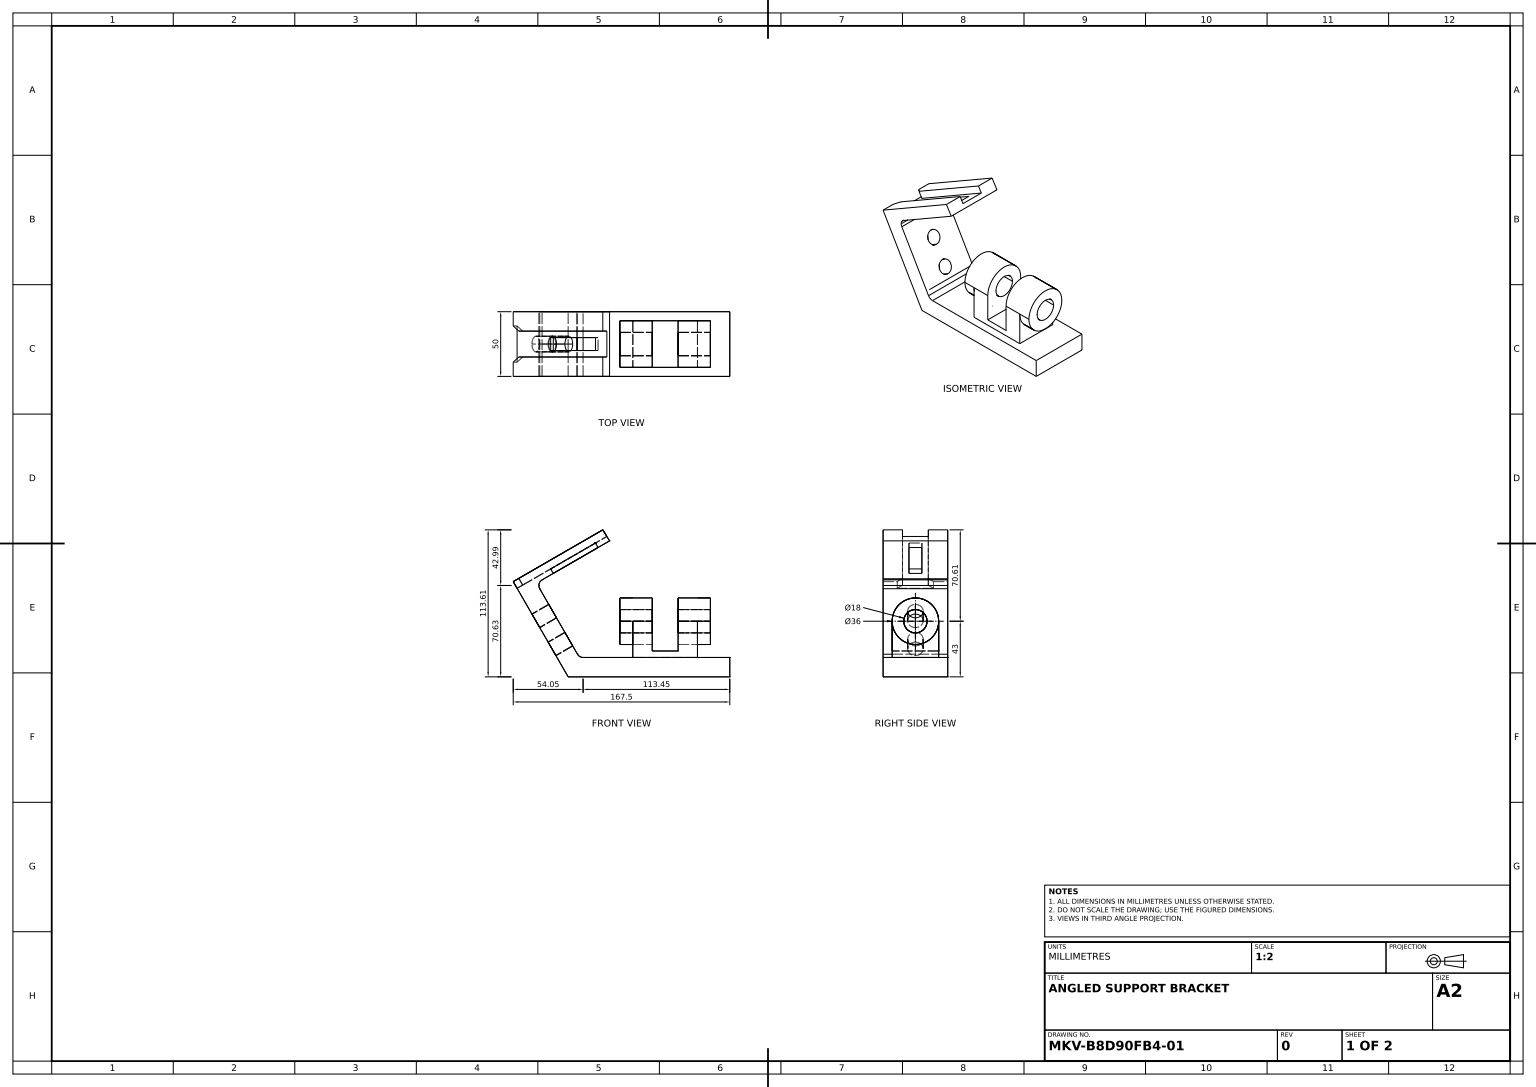
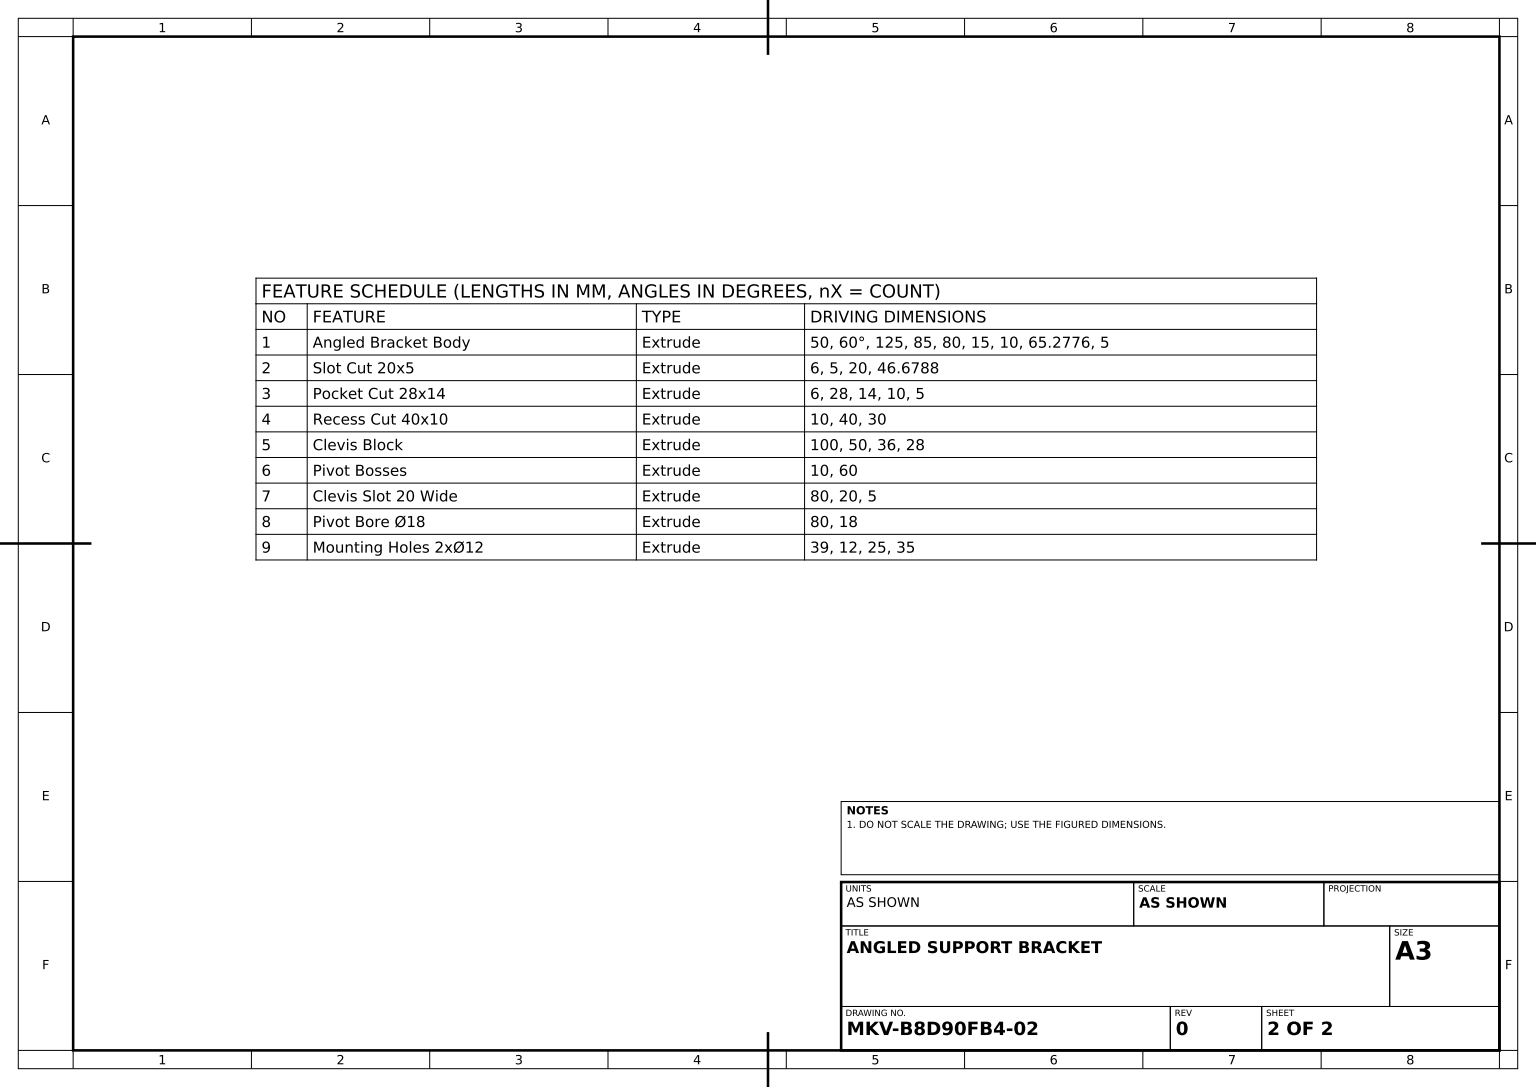
from build123d import *

# Parameters (mm, degrees)
ANGLED_BRACKET_BODY_DEPTH  = 25
SLOT_20X5_SKETCH_W         = 83.357534166
SLOT_20X5_SKETCH_H         = 20
SLOT_CUT_20X5_DEPTH        = 6
POCKET_CUT_28X14_DEPTH     = 6
RECESS_40X10_SKETCH_W      = 40
RECESS_40X10_SKETCH_H      = 10
RECESS_CUT_40X10_DEPTH     = 10
CLEVIS_BLOCK_SKETCH_W      = 36
CLEVIS_BLOCK_SKETCH_H      = 28
CLEVIS_BLOCK_DEPTH         = 50
PIVOT_BOSSES_DEPTH         = 10
PIVOT_BOSSES_DEPTH_BACK    = 60
PIVOT_BOSS_SKETCH_R        = 18
CLEVIS_SLOT_SKETCH_W       = 20
CLEVIS_SLOT_SKETCH_H       = 46
CLEVIS_SLOT_20_WIDE_DEPTH  = 80
PIVOT_BORE_SKETCH_R        = 9
PIVOT_BORE_18_DEPTH        = 80
MOUNTING_HOLES_SKETCH_R    = 6
MOUNTING_HOLES_2X_12_DEPTH = 39


with BuildPart() as part:
    # Bracket Profile Sketch → Angled Bracket Body (new, symmetric)
    with BuildSketch(Plane.XY):
        with BuildLine():
            Line((125, 0), (0, 0))
            Line((0, 0), (-42.5, 73.612159322))
            Line((-42.5, 73.612159322), (26.782032303, 113.612159322))
            Line((26.782032303, 113.612159322), (32.020529704, 105.094052432))
            Line((32.020529704, 105.094052432), (-20.181419095, 74.955243241))
            ThreePointArc((-20.181419095, 74.955243241), (-22.511048226, 71.919211448), (-22.011546114, 68.125116222))
            Line((-22.011546114, 68.125116222), (7.216878365, 17.5))
            ThreePointArc((7.216878365, 17.5), (9.047005384, 15.669872981), (11.547005384, 15))
            Line((11.547005384, 15), (125, 15))
            Line((125, 15), (125, 0))
        make_face()
    extrude(amount=ANGLED_BRACKET_BODY_DEPTH, both=True)

    # Slot 20x5 Sketch → Slot Cut 20x5 (cut)
    with BuildSketch(Plane(origin=(-42.5, 73.612159322, 0), x_dir=(0.8660254037844364, 0.5000000000000041, 0), z_dir=(-0.5000000000000041, 0.8660254037844364, 0))):
        with Locations((46.678767083, 0)):
            Rectangle(SLOT_20X5_SKETCH_W, SLOT_20X5_SKETCH_H)
    extrude(amount=-SLOT_CUT_20X5_DEPTH, mode=Mode.SUBTRACT)

    # Pocket 28x14 Sketch → Pocket Cut 28x14 (cut)
    with BuildSketch(Plane(origin=(-42.5, 73.612159322, 0), x_dir=(0.8660254037844364, 0.5000000000000041, 0), z_dir=(-0.5000000000000041, 0.8660254037844364, 0))):
        Polygon((0, 14), (0, -14), (5, -10), (5, 10), align=None)
    extrude(amount=-POCKET_CUT_28X14_DEPTH, mode=Mode.SUBTRACT)

    # Recess 40x10 Sketch → Recess Cut 40x10 (cut)
    with BuildSketch(Plane(origin=(-39.5, 68.416006899, 0), x_dir=(0.8660254037844364, 0.5000000000000041, 0), z_dir=(-0.500000000000004, 0.8660254037844363, 0))):
        with Locations((50, 0)):
            Rectangle(RECESS_40X10_SKETCH_W, RECESS_40X10_SKETCH_H)
    extrude(amount=-RECESS_CUT_40X10_DEPTH, mode=Mode.SUBTRACT)

    # Clevis Block Sketch → Clevis Block (add)
    with BuildSketch(Plane(origin=(100, 0, 0), x_dir=(0, 0, -1), z_dir=(1, 0, 0))):
        with Locations((0, 29)):
            Rectangle(CLEVIS_BLOCK_SKETCH_W, CLEVIS_BLOCK_SKETCH_H)
    extrude(amount=-CLEVIS_BLOCK_DEPTH)

    # Pivot Boss Sketch → Pivot Bosses (add, two sides: drawn at the far end of the back side and taken through both)
    with BuildSketch(Plane(origin=(100, 0, 0), x_dir=(0, 0, -1), z_dir=(1, 0, 0)).offset(-PIVOT_BOSSES_DEPTH_BACK)):
        with Locations((0, 43)):
            Circle(PIVOT_BOSS_SKETCH_R)
    extrude(amount=PIVOT_BOSSES_DEPTH + PIVOT_BOSSES_DEPTH_BACK)

    # Clevis Slot Sketch → Clevis Slot 20 Wide (cut)
    with BuildSketch(Plane.XY.offset(18)):
        with Locations((75, 43)):
            Rectangle(CLEVIS_SLOT_SKETCH_W, CLEVIS_SLOT_SKETCH_H)
    extrude(amount=-CLEVIS_SLOT_20_WIDE_DEPTH, mode=Mode.SUBTRACT)

    # Pivot Bore Sketch → Pivot Bore Ø18 (cut)
    with BuildSketch(Plane(origin=(110, 0, 0), x_dir=(0, 0, -1), z_dir=(1, 0, 0))):
        with Locations((0, 43)):
            Circle(PIVOT_BORE_SKETCH_R)
    extrude(amount=-PIVOT_BORE_18_DEPTH, mode=Mode.SUBTRACT)

    # Mounting Holes Sketch → Mounting Holes 2xØ12 (cut)
    with BuildSketch(Plane(origin=(0, 0, 0), x_dir=(0, 0, 1), z_dir=(-0.8660254037844363, -0.5000000000000042, 0))):
        with Locations(Location((0, 50, 0), (0, 0, 270))):
            Circle(MOUNTING_HOLES_SKETCH_R)
        with Locations(Location((0, 25, 0), (0, 0, 270))):
            Circle(MOUNTING_HOLES_SKETCH_R)
    extrude(amount=-MOUNTING_HOLES_2X_12_DEPTH, mode=Mode.SUBTRACT)


solid = part.part
